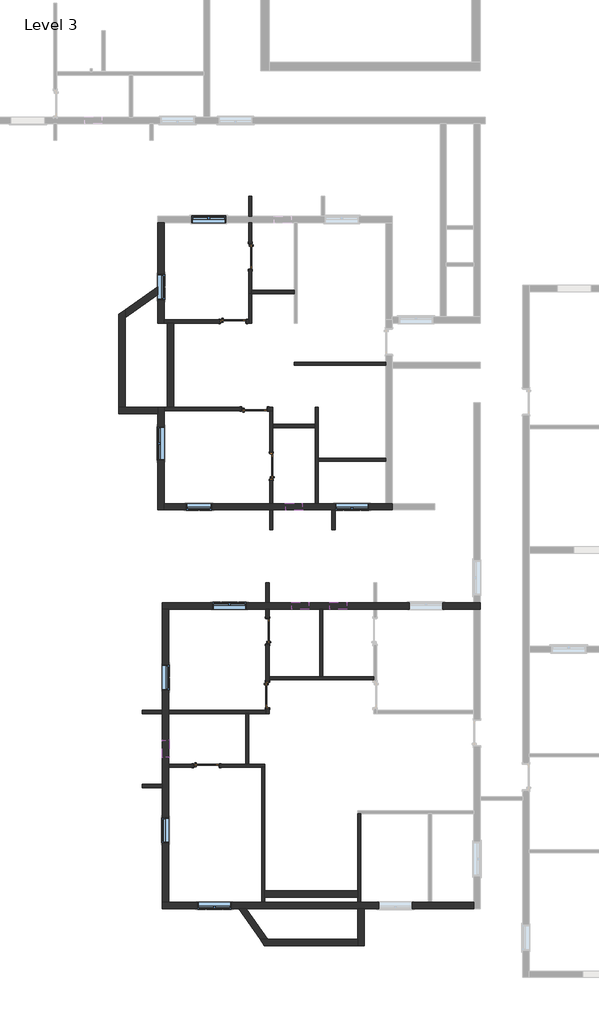
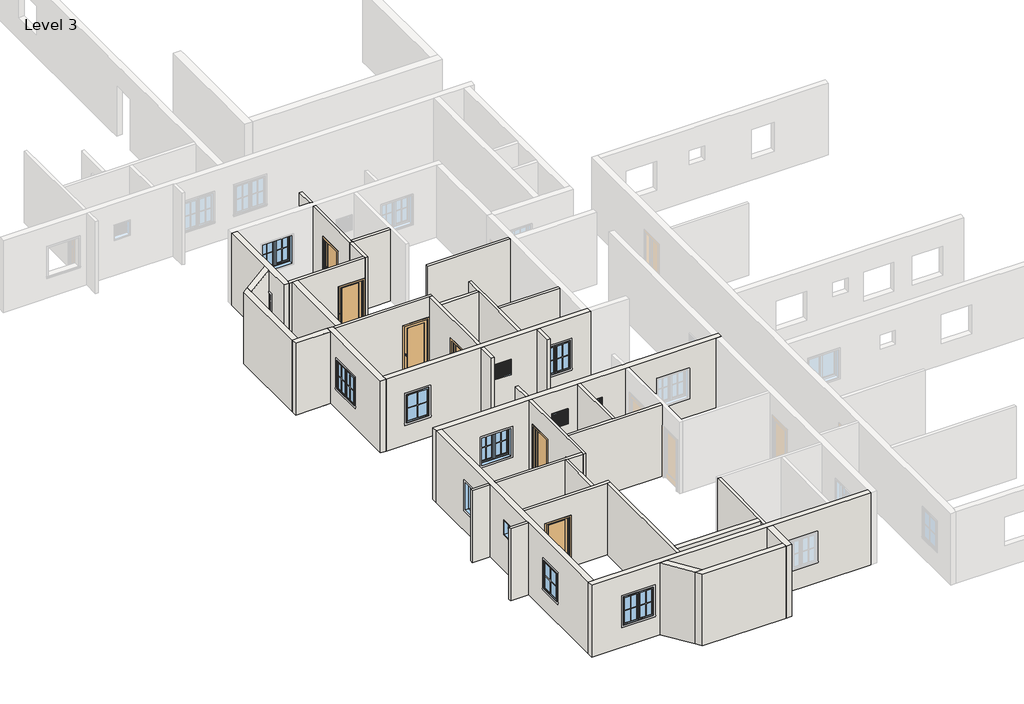
# One storey, part 1 of 7: 39 walls, 13 windows, 7 doors.
"""IFC4 building model written with IfcOpenShell, lengths in millimetres."""

from ifc_helpers import new_model, si_unit, frame, origin, place, context, project, spatial, polyline, outline, extrude, faceted_brep, transform, mapped, element, save
from components import door_3c6ab76a, door_a3feeac7, window_272f20d6, window_casement_double_4_x_4_af3140d2, window_f2d8fef0

model = new_model("IFC4")

# Units and contexts
model_context = context("Model", 3, world=origin())
ifc_project = project(units=[si_unit("LENGTHUNIT", "METRE", prefix="MILLI")], contexts=[model_context])

# Site, building, storey
site = spatial("IfcSite", under=ifc_project)
building = spatial("IfcBuilding", under=site)
storey = spatial("IfcBuildingStorey", under=building, Name="Level 3", Elevation=3200.4)

# Doors
placement = place(None, origin())
door_shape = door_3c6ab76a(model_context)
element("IfcDoor", 1, ObjectType="Door-Interior-Single-1_Panel-Wood : 2'6\" x 7' door", at=placement, inside=storey, context=model_context, shape_type="MappedRepresentation", body=[
    mapped(door_shape, transform((-4216.6759469, -3460.4538828, 3200.4), x_axis=(0.0, -1.0, 0.0), y_axis=(1.0, 0.0, 0.0), z_axis=(0.0, 0.0, 1.0))),
])
element("IfcDoor", 2, ObjectType="Door-Interior-Single-1_Panel-Wood : 2'6\" x 7' door", at=placement, inside=storey, context=model_context, shape_type="MappedRepresentation", body=[
    mapped(door_shape, transform((-5797.8259469, -21840.5288828, 3200.4), x_axis=(1.0, 0.0, 0.0), y_axis=(0.0, 1.0, 0.0), z_axis=(0.0, 0.0, 1.0))),
])
door_2_shape = door_a3feeac7(model_context)
element("IfcDoor", 3, ObjectType="Door-Interior-Single-1_Panel-Wood : 2'6\" x 7' door", at=placement, inside=storey, context=model_context, shape_type="MappedRepresentation", body=[
    mapped(door_2_shape, transform((-3454.6759469, -11032.8288828, 3200.4), x_axis=(0.0, 1.0, 0.0), y_axis=(-1.0, 0.0, 0.0), z_axis=(0.0, 0.0, 1.0))),
])
element("IfcDoor", 4, ObjectType="Door-Interior-Single-1_Panel-Wood : 2'6\" x 7' door", at=placement, inside=storey, context=model_context, shape_type="MappedRepresentation", body=[
    mapped(door_2_shape, transform((-3594.3759469, -16985.9538828, 3200.4), x_axis=(0.0, 1.0, 0.0), y_axis=(-1.0, 0.0, 0.0), z_axis=(0.0, 0.0, 1.0))),
])
element("IfcDoor", 5, ObjectType="Door-Interior-Single-1_Panel-Wood : 36\" x 84\"", at=placement, inside=storey, context=model_context, shape_type="MappedRepresentation", body=[
    mapped(door_shape, transform((-4829.4509469, -5800.4288828, 3200.4), x_axis=(1.0, 0.0, 0.0), y_axis=(0.0, 1.0, 0.0), z_axis=(0.0, 0.0, 1.0))),
])
element("IfcDoor", 6, ObjectType="Door-Interior-Single-1_Panel-Wood : 36\" x 84\"", at=placement, inside=storey, context=model_context, shape_type="MappedRepresentation", body=[
    mapped(door_2_shape, transform((-4067.4509469, -8969.0788828, 3200.4), x_axis=(1.0, 0.0, 0.0), y_axis=(0.0, 1.0, 0.0), z_axis=(0.0, 0.0, 1.0))),
])
element("IfcDoor", 7, ObjectType="Door-Interior-Single-1_Panel-Wood : 36\" x 84\"", at=placement, inside=storey, context=model_context, shape_type="MappedRepresentation", body=[
    mapped(door_2_shape, transform((-3600.7259469, -19291.0038828, 3200.4), x_axis=(0.0, -1.0, 0.0), y_axis=(1.0, 0.0, 0.0), z_axis=(0.0, 0.0, 1.0))),
])

# Walls
element("IfcWall", 8, ObjectType="4.5\" wall", at=placement, inside=storey, context=model_context, shape_type="Brep", body=[
    faceted_brep([(-4277.0009469, -4793.9538828, 6248.4), (-4277.0009469, -2241.2538828, 6248.4), (-4277.0009469, -2241.2538828, 3200.4), (-4277.0009469, -2977.8538828, 3200.4), (-4277.0009469, -2977.8538828, 5359.4), (-4277.0009469, -3943.0538828, 5359.4), (-4277.0009469, -3943.0538828, 3200.4), (-4277.0009469, -4793.9538828, 3200.4), (-4162.7009469, -2241.2538828, 6248.4), (-4162.7009469, -4679.6538828, 6248.4), (-4162.7009469, -4793.9538828, 6248.4), (-4162.7009469, -4793.9538828, 3200.4), (-4162.7009469, -4679.6538828, 3200.4), (-4162.7009469, -3943.0538828, 3200.4), (-4162.7009469, -3943.0538828, 5359.4), (-4162.7009469, -2977.8538828, 5359.4), (-4162.7009469, -2977.8538828, 3200.4), (-4162.7009469, -2241.2538828, 3200.4)], [[[0, 1, 2, 3, 4, 5, 6, 7]], [[8, 9, 10, 11, 12, 13, 14, 15, 16, 17]], [[2, 17, 16, 3]], [[11, 7, 6, 13, 12]], [[1, 0, 10, 9, 8]], [[2, 1, 8, 17]], [[0, 7, 11, 10]], [[5, 14, 13, 6]], [[14, 5, 4, 15]], [[15, 4, 3, 16]]]),
])
element("IfcWall", 9, ObjectType="4.5\" wall", at=placement, inside=storey, context=model_context, shape_type="Brep", body=[
    faceted_brep([(-4277.0009469, -4793.9538828, 3200.4), (-4277.0009469, -5746.4538828, 3200.4), (-4277.0009469, -5860.7538828, 3200.4), (-4277.0009469, -5860.7538828, 6248.4), (-4277.0009469, -5746.4538828, 6248.4), (-4277.0009469, -4793.9538828, 6248.4), (-4162.7009469, -4793.9538828, 3200.4), (-4162.7009469, -4793.9538828, 6248.4), (-4162.7009469, -5860.7538828, 6248.4), (-4162.7009469, -5860.7538828, 3200.4)], [[[0, 1, 2, 3, 4, 5]], [[6, 7, 8, 9]], [[2, 1, 0, 6, 9]], [[5, 4, 3, 8, 7]], [[0, 5, 7, 6]], [[3, 2, 9, 8]]]),
])
element("IfcWall", 10, ObjectType="4.5\" wall", at=placement, inside=storey, context=model_context, shape_type="Brep", body=[
    faceted_brep([(-7325.0009469, -5746.4538828, 6248.4), (-4277.0009469, -5746.4538828, 6248.4), (-4277.0009469, -5746.4538828, 3200.4), (-4346.8509469, -5746.4538828, 3200.4), (-4346.8509469, -5746.4538828, 5359.4), (-5312.0509469, -5746.4538828, 5359.4), (-5312.0509469, -5746.4538828, 3200.4), (-7325.0009469, -5746.4538828, 3200.4), (-4277.0009469, -5860.7538828, 6248.4), (-6982.1009469, -5860.7538828, 6248.4), (-7210.7009469, -5860.7538828, 6248.4), (-7325.0009469, -5860.7538828, 6248.4), (-7325.0009469, -5860.7538828, 3200.4), (-7210.7009469, -5860.7538828, 3200.4), (-6982.1009469, -5860.7538828, 3200.4), (-5312.0509469, -5860.7538828, 3200.4), (-5312.0509469, -5860.7538828, 5359.4), (-4346.8509469, -5860.7538828, 5359.4), (-4346.8509469, -5860.7538828, 3200.4), (-4277.0009469, -5860.7538828, 3200.4)], [[[0, 1, 2, 3, 4, 5, 6, 7]], [[8, 9, 10, 11, 12, 13, 14, 15, 16, 17, 18, 19]], [[12, 7, 6, 15, 14, 13]], [[2, 19, 18, 3]], [[1, 0, 11, 10, 9, 8]], [[0, 7, 12, 11]], [[2, 1, 8, 19]], [[17, 4, 3, 18]], [[4, 17, 16, 5]], [[5, 16, 15, 6]]]),
])
element("IfcWall", 11, ObjectType="4.5\" wall", at=placement, inside=storey, context=model_context, shape_type="SweptSolid", body=[
    extrude(outline(polyline([(-2638.7009469, -4793.9538828), (-4162.7009469, -4793.9538828), (-4162.7009469, -4679.6538828), (-2638.7009469, -4679.6538828), (-2638.7009469, -4793.9538828)])), frame((0.0, 0.0, 3200.4), z_axis=(0.0, 0.0, 1.0), x_axis=(1.0, 0.0, 0.0)), (0.0, 0.0, 1.0), 3048.0),
])
element("IfcWall", 12, ObjectType="4.5\" wall", at=placement, inside=storey, context=model_context, shape_type="SweptSolid", body=[
    extrude(outline(polyline([(-2638.7009469, -7270.4538828), (675.9990531, -7270.4538828), (675.9990531, -7384.7538828), (-2638.7009469, -7384.7538828), (-2638.7009469, -7270.4538828)])), frame((0.0, 0.0, 3200.4), z_axis=(0.0, 0.0, 1.0), x_axis=(1.0, 0.0, 0.0)), (0.0, 0.0, 1.0), 3048.0),
])
element("IfcWall", 13, ObjectType="4.5\" wall", at=placement, inside=storey, context=model_context, shape_type="Brep", body=[
    faceted_brep([(-7325.0009469, -8908.7538828, 6248.4), (-7210.7009469, -8908.7538828, 6248.4), (-6982.1009469, -8908.7538828, 6248.4), (-3400.7009469, -8908.7538828, 6248.4), (-3400.7009469, -8908.7538828, 3200.4), (-3584.8509469, -8908.7538828, 3200.4), (-3584.8509469, -8908.7538828, 5359.4), (-4550.0509469, -8908.7538828, 5359.4), (-4550.0509469, -8908.7538828, 3200.4), (-6982.1009469, -8908.7538828, 3200.4), (-7210.7009469, -8908.7538828, 3200.4), (-7325.0009469, -8908.7538828, 3200.4), (-3400.7009469, -9023.0538828, 6248.4), (-3515.0009469, -9023.0538828, 6248.4), (-7325.0009469, -9023.0538828, 6248.4), (-7325.0009469, -9023.0538828, 3200.4), (-4550.0509469, -9023.0538828, 3200.4), (-4550.0509469, -9023.0538828, 5359.4), (-3584.8509469, -9023.0538828, 5359.4), (-3584.8509469, -9023.0538828, 3200.4), (-3515.0009469, -9023.0538828, 3200.4), (-3400.7009469, -9023.0538828, 3200.4)], [[[0, 1, 2, 3, 4, 5, 6, 7, 8, 9, 10, 11]], [[12, 13, 14, 15, 16, 17, 18, 19, 20, 21]], [[4, 21, 20, 19, 5]], [[15, 11, 10, 9, 8, 16]], [[3, 2, 1, 0, 14, 13, 12]], [[4, 3, 12, 21]], [[0, 11, 15, 14]], [[18, 6, 5, 19]], [[6, 18, 17, 7]], [[7, 17, 16, 8]]]),
])
element("IfcWall", 14, ObjectType="4.5\" wall", at=placement, inside=storey, context=model_context, shape_type="SweptSolid", body=[
    extrude(outline(polyline([(-1876.7009469, -9632.6538828), (-3400.7009469, -9632.6538828), (-3400.7009469, -9518.3538828), (-1876.7009469, -9518.3538828), (-1876.7009469, -9632.6538828)])), frame((0.0, 0.0, 3200.4), z_axis=(0.0, 0.0, 1.0), x_axis=(1.0, 0.0, 0.0)), (0.0, 0.0, 1.0), 3048.0),
])
element("IfcWall", 15, ObjectType="4.5\" wall", at=placement, inside=storey, context=model_context, shape_type="Brep", body=[
    faceted_brep([(-1762.4009469, -12375.8538828, 3200.4), (-1762.4009469, -10851.8538828, 3200.4), (-1762.4009469, -10737.5538828, 3200.4), (-1762.4009469, -8908.7538828, 3200.4), (-1762.4009469, -8908.7538828, 6248.4), (-1762.4009469, -10737.5538828, 6248.4), (-1762.4009469, -10851.8538828, 6248.4), (-1762.4009469, -12375.8538828, 6248.4), (-1876.7009469, -12375.8538828, 3200.4), (-1876.7009469, -12375.8538828, 6248.4), (-1876.7009469, -9632.6538828, 6248.4), (-1876.7009469, -9518.3538828, 6248.4), (-1876.7009469, -8908.7538828, 6248.4), (-1876.7009469, -8908.7538828, 3200.4), (-1876.7009469, -9518.3538828, 3200.4), (-1876.7009469, -9632.6538828, 3200.4)], [[[0, 1, 2, 3, 4, 5, 6, 7]], [[8, 9, 10, 11, 12, 13, 14, 15]], [[3, 2, 1, 0, 8, 15, 14, 13]], [[4, 3, 13, 12]], [[7, 6, 5, 4, 12, 11, 10, 9]], [[0, 7, 9, 8]]]),
])
element("IfcWall", 16, ObjectType="4.5\" wall", at=placement, inside=storey, context=model_context, shape_type="Brep", body=[
    faceted_brep([(-3400.7009469, -9023.0538828, 6248.4), (-3400.7009469, -9518.3538828, 6248.4), (-3400.7009469, -9632.6538828, 6248.4), (-3400.7009469, -12375.8538828, 6248.4), (-3400.7009469, -12375.8538828, 3200.4), (-3400.7009469, -11515.4288828, 3200.4), (-3400.7009469, -11515.4288828, 5359.4), (-3400.7009469, -10550.2288828, 5359.4), (-3400.7009469, -10550.2288828, 3200.4), (-3400.7009469, -9632.6538828, 3200.4), (-3400.7009469, -9518.3538828, 3200.4), (-3400.7009469, -9023.0538828, 3200.4), (-3515.0009469, -12375.8538828, 6248.4), (-3515.0009469, -9023.0538828, 6248.4), (-3515.0009469, -9023.0538828, 3200.4), (-3515.0009469, -10550.2288828, 3200.4), (-3515.0009469, -10550.2288828, 5359.4), (-3515.0009469, -11515.4288828, 5359.4), (-3515.0009469, -11515.4288828, 3200.4), (-3515.0009469, -12375.8538828, 3200.4)], [[[0, 1, 2, 3, 4, 5, 6, 7, 8, 9, 10, 11]], [[12, 13, 14, 15, 16, 17, 18, 19]], [[4, 19, 18, 5]], [[14, 11, 10, 9, 8, 15]], [[3, 2, 1, 0, 13, 12]], [[4, 3, 12, 19]], [[0, 11, 14, 13]], [[7, 16, 15, 8]], [[16, 7, 6, 17]], [[17, 6, 5, 18]]]),
])
element("IfcWall", 17, ObjectType="4.5\" wall", at=placement, inside=storey, context=model_context, shape_type="SweptSolid", body=[
    extrude(outline(polyline([(-1762.4009469, -10737.5538828), (675.9990531, -10737.5538828), (675.9990531, -10851.8538828), (-1762.4009469, -10851.8538828), (-1762.4009469, -10737.5538828)])), frame((0.0, 0.0, 3200.4), z_axis=(0.0, 0.0, 1.0), x_axis=(1.0, 0.0, 0.0)), (0.0, 0.0, 1.0), 3048.0),
])
element("IfcWall", 18, ObjectType="4.5\" wall", at=placement, inside=storey, context=model_context, shape_type="SweptSolid", body=[
    extrude(outline(polyline([(-3515.0009469, -13328.3538828), (-3515.0009469, -12604.4538828), (-3400.7009469, -12604.4538828), (-3400.7009469, -13328.3538828), (-3515.0009469, -13328.3538828)])), frame((0.0, 0.0, 3200.4), z_axis=(0.0, 0.0, 1.0), x_axis=(1.0, 0.0, 0.0)), (0.0, 0.0, 1.0), 3048.0),
])
element("IfcWall", 19, ObjectType="4.5\" wall", at=placement, inside=storey, context=model_context, shape_type="SweptSolid", body=[
    extrude(outline(polyline([(-1152.8009469, -12604.4538828), (-1152.8009469, -13328.3538828), (-1267.1009469, -13328.3538828), (-1267.1009469, -12604.4538828), (-1152.8009469, -12604.4538828)])), frame((0.0, 0.0, 3200.4), z_axis=(0.0, 0.0, 1.0), x_axis=(1.0, 0.0, 0.0)), (0.0, 0.0, 1.0), 3048.0),
])
element("IfcWall", 20, ObjectType="4.5\" wall", at=placement, inside=storey, context=model_context, shape_type="SweptSolid", body=[
    extrude(outline(polyline([(-4162.7009469, -1288.7538828), (-4162.7009469, -2012.6538828), (-4277.0009469, -2012.6538828), (-4277.0009469, -1288.7538828), (-4162.7009469, -1288.7538828)])), frame((0.0, 0.0, 3200.4), z_axis=(0.0, 0.0, 1.0), x_axis=(1.0, 0.0, 0.0)), (0.0, 0.0, 1.0), 3048.0),
])
element("IfcWall", 21, ObjectType="4.5\" wall", at=placement, inside=storey, context=model_context, shape_type="Brep", body=[
    faceted_brep([(231.4990531, -18624.2538828, 3200.4), (-1597.3009469, -18624.2538828, 3200.4), (-1711.6009469, -18624.2538828, 3200.4), (-3540.4009469, -18624.2538828, 3200.4), (-3540.4009469, -18624.2538828, 6248.4), (-1711.6009469, -18624.2538828, 6248.4), (-1597.3009469, -18624.2538828, 6248.4), (231.4990531, -18624.2538828, 6248.4), (231.4990531, -18738.5538828, 3200.4), (231.4990531, -18738.5538828, 6248.4), (-3540.4009469, -18738.5538828, 6248.4), (-3540.4009469, -18738.5538828, 3200.4)], [[[0, 1, 2, 3, 4, 5, 6, 7]], [[8, 9, 10, 11]], [[3, 2, 1, 0, 8, 11]], [[7, 6, 5, 4, 10, 9]], [[4, 3, 11, 10]], [[0, 7, 9, 8]]]),
])
element("IfcWall", 22, ObjectType="4.5\" wall", at=placement, inside=storey, context=model_context, shape_type="SweptSolid", body=[
    extrude(outline(polyline([(-1597.3009469, -16185.8538828), (-1597.3009469, -18624.2538828), (-1711.6009469, -18624.2538828), (-1711.6009469, -16185.8538828), (-1597.3009469, -16185.8538828)])), frame((0.0, 0.0, 3200.4), z_axis=(0.0, 0.0, 1.0), x_axis=(1.0, 0.0, 0.0)), (0.0, 0.0, 1.0), 3048.0),
])
element("IfcWall", 23, ObjectType="4.5\" wall", at=placement, inside=storey, context=model_context, shape_type="SweptSolid", body=[
    extrude(outline(polyline([(-3540.4009469, -15233.3538828), (-3540.4009469, -15957.2538828), (-3654.7009469, -15957.2538828), (-3654.7009469, -15233.3538828), (-3540.4009469, -15233.3538828)])), frame((0.0, 0.0, 3200.4), z_axis=(0.0, 0.0, 1.0), x_axis=(1.0, 0.0, 0.0)), (0.0, 0.0, 1.0), 3048.0),
])
element("IfcWall", 24, ObjectType="4.5\" wall", at=placement, inside=storey, context=model_context, shape_type="Brep", body=[
    faceted_brep([(-3654.7009469, -19957.7538828, 6248.4), (-3654.7009469, -19843.4538828, 6248.4), (-3654.7009469, -16185.8538828, 6248.4), (-3654.7009469, -16185.8538828, 3200.4), (-3654.7009469, -16503.3538828, 3200.4), (-3654.7009469, -16503.3538828, 5359.4), (-3654.7009469, -17468.5538828, 5359.4), (-3654.7009469, -17468.5538828, 3200.4), (-3654.7009469, -18808.4038828, 3200.4), (-3654.7009469, -18808.4038828, 5359.4), (-3654.7009469, -19773.6038828, 5359.4), (-3654.7009469, -19773.6038828, 3200.4), (-3654.7009469, -19843.4538828, 3200.4), (-3654.7009469, -19957.7538828, 3200.4), (-3540.4009469, -16185.8538828, 6248.4), (-3540.4009469, -18624.2538828, 6248.4), (-3540.4009469, -18738.5538828, 6248.4), (-3540.4009469, -19957.7538828, 6248.4), (-3540.4009469, -19957.7538828, 3200.4), (-3540.4009469, -19773.6038828, 3200.4), (-3540.4009469, -19773.6038828, 5359.4), (-3540.4009469, -18808.4038828, 5359.4), (-3540.4009469, -18808.4038828, 3200.4), (-3540.4009469, -18738.5538828, 3200.4), (-3540.4009469, -18624.2538828, 3200.4), (-3540.4009469, -17468.5538828, 3200.4), (-3540.4009469, -17468.5538828, 5359.4), (-3540.4009469, -16503.3538828, 5359.4), (-3540.4009469, -16503.3538828, 3200.4), (-3540.4009469, -16185.8538828, 3200.4)], [[[0, 1, 2, 3, 4, 5, 6, 7, 8, 9, 10, 11, 12, 13]], [[14, 15, 16, 17, 18, 19, 20, 21, 22, 23, 24, 25, 26, 27, 28, 29]], [[3, 29, 28, 4]], [[18, 13, 12, 11, 19]], [[7, 25, 24, 23, 22, 8]], [[2, 1, 0, 17, 16, 15, 14]], [[3, 2, 14, 29]], [[0, 13, 18, 17]], [[27, 5, 4, 28]], [[5, 27, 26, 6]], [[6, 26, 25, 7]], [[10, 20, 19, 11]], [[20, 10, 9, 21]], [[21, 9, 8, 22]]]),
])
element("IfcWall", 25, ObjectType="4.5\" wall", at=placement, inside=storey, context=model_context, shape_type="Brep", body=[
    faceted_brep([(-3654.7009469, -19843.4538828, 3200.4), (-7159.9009469, -19843.4538828, 3200.4), (-7159.9009469, -19843.4538828, 6248.4), (-3654.7009469, -19843.4538828, 6248.4), (-3654.7009469, -19957.7538828, 3200.4), (-3654.7009469, -19957.7538828, 6248.4), (-4264.3009469, -19957.7538828, 6248.4), (-4378.6009469, -19957.7538828, 6248.4), (-7159.9009469, -19957.7538828, 6248.4), (-7159.9009469, -19957.7538828, 3200.4), (-4378.6009469, -19957.7538828, 3200.4), (-4264.3009469, -19957.7538828, 3200.4)], [[[0, 1, 2, 3]], [[4, 5, 6, 7, 8, 9, 10, 11]], [[1, 0, 4, 11, 10, 9]], [[3, 2, 8, 7, 6, 5]], [[2, 1, 9, 8]], [[0, 3, 5, 4]]]),
])
element("IfcWall", 26, ObjectType="4.5\" wall", at=placement, inside=storey, context=model_context, shape_type="Brep", body=[
    faceted_brep([(-7159.9009469, -21786.5538828, 6248.4), (-4378.6009469, -21786.5538828, 6248.4), (-4264.3009469, -21786.5538828, 6248.4), (-3692.8009469, -21786.5538828, 6248.4), (-3692.8009469, -21786.5538828, 3200.4), (-4264.3009469, -21786.5538828, 3200.4), (-4378.6009469, -21786.5538828, 3200.4), (-5315.2259469, -21786.5538828, 3200.4), (-5315.2259469, -21786.5538828, 5359.4), (-6280.4259469, -21786.5538828, 5359.4), (-6280.4259469, -21786.5538828, 3200.4), (-7159.9009469, -21786.5538828, 3200.4), (-3692.8009469, -21900.8538828, 6248.4), (-3807.1009469, -21900.8538828, 6248.4), (-7159.9009469, -21900.8538828, 6248.4), (-7159.9009469, -21900.8538828, 3200.4), (-6280.4259469, -21900.8538828, 3200.4), (-6280.4259469, -21900.8538828, 5359.4), (-5315.2259469, -21900.8538828, 5359.4), (-5315.2259469, -21900.8538828, 3200.4), (-3807.1009469, -21900.8538828, 3200.4), (-3692.8009469, -21900.8538828, 3200.4)], [[[0, 1, 2, 3, 4, 5, 6, 7, 8, 9, 10, 11]], [[12, 13, 14, 15, 16, 17, 18, 19, 20, 21]], [[15, 11, 10, 16]], [[4, 21, 20, 19, 7, 6, 5]], [[3, 2, 1, 0, 14, 13, 12]], [[0, 11, 15, 14]], [[4, 3, 12, 21]], [[18, 8, 7, 19]], [[8, 18, 17, 9]], [[9, 17, 16, 10]]]),
])
element("IfcWall", 27, ObjectType="4.5\" wall", at=placement, inside=storey, context=model_context, shape_type="Brep", body=[
    faceted_brep([(-3692.8009469, -26777.6538828, 3200.4), (-3692.8009469, -26587.1538828, 3200.4), (-3692.8009469, -26358.5538828, 3200.4), (-3692.8009469, -21900.8538828, 3200.4), (-3692.8009469, -21900.8538828, 6248.4), (-3692.8009469, -26358.5538828, 6248.4), (-3692.8009469, -26587.1538828, 6248.4), (-3692.8009469, -26777.6538828, 6248.4), (-3807.1009469, -26777.6538828, 3200.4), (-3807.1009469, -26777.6538828, 6248.4), (-3807.1009469, -21900.8538828, 6248.4), (-3807.1009469, -21900.8538828, 3200.4)], [[[0, 1, 2, 3, 4, 5, 6, 7]], [[8, 9, 10, 11]], [[3, 2, 1, 0, 8, 11]], [[7, 6, 5, 4, 10, 9]], [[4, 3, 11, 10]], [[0, 7, 9, 8]]]),
])
element("IfcWall", 28, ObjectType="4.5\" wall", at=placement, inside=storey, context=model_context, shape_type="SweptSolid", body=[
    extrude(outline(polyline([(-7388.5009469, -22629.8863256), (-8112.4009469, -22629.8863256), (-8112.4009469, -22515.5863256), (-7388.5009469, -22515.5863256), (-7388.5009469, -22629.8863256)])), frame((0.0, 0.0, 3200.4), z_axis=(0.0, 0.0, 1.0), x_axis=(1.0, 0.0, 0.0)), (0.0, 0.0, 1.0), 3048.0),
])
element("IfcWall", 29, ObjectType="4.5\" wall", at=placement, inside=storey, context=model_context, shape_type="SweptSolid", body=[
    extrude(outline(polyline([(-8112.4009469, -19843.4538828), (-7388.5009469, -19843.4538828), (-7388.5009469, -19957.7538828), (-8112.4009469, -19957.7538828), (-8112.4009469, -19843.4538828)])), frame((0.0, 0.0, 3200.4), z_axis=(0.0, 0.0, 1.0), x_axis=(1.0, 0.0, 0.0)), (0.0, 0.0, 1.0), 3048.0),
])
element("IfcWall", 30, ObjectType="4.5\" wall", at=placement, inside=storey, context=model_context, shape_type="SweptSolid", body=[
    extrude(outline(polyline([(-4378.6009469, -21786.5538828), (-4378.6009469, -19957.7538828), (-4264.3009469, -19957.7538828), (-4264.3009469, -21786.5538828), (-4378.6009469, -21786.5538828)])), frame((0.0, 0.0, 3200.4), z_axis=(0.0, 0.0, 1.0), x_axis=(1.0, 0.0, 0.0)), (0.0, 0.0, 1.0), 3048.0),
])
element("IfcWall", 31, ObjectType="4.5\" wall", at=placement, inside=storey, context=model_context, shape_type="Brep", body=[
    faceted_brep([(-340.0009469, -23577.2538828, 3200.4), (-340.0009469, -26358.5538828, 3200.4), (-340.0009469, -26587.1538828, 3200.4), (-340.0009469, -26777.6538828, 3200.4), (-340.0009469, -26777.6538828, 6248.4), (-340.0009469, -26587.1538828, 6248.4), (-340.0009469, -26358.5538828, 6248.4), (-340.0009469, -23577.2538828, 6248.4), (-225.7009469, -23577.2538828, 3200.4), (-225.7009469, -23577.2538828, 6248.4), (-225.7009469, -26777.6538828, 6248.4), (-225.7009469, -26777.6538828, 3200.4)], [[[0, 1, 2, 3, 4, 5, 6, 7]], [[8, 9, 10, 11]], [[3, 2, 1, 0, 8, 11]], [[7, 6, 5, 4, 10, 9]], [[0, 7, 9, 8]], [[4, 3, 11, 10]]]),
])
element("IfcWall", 32, ObjectType="9\"", at=placement, inside=storey, context=model_context, shape_type="Brep", body=[
    faceted_brep([(-7553.6009469, -2241.2538828, 3200.4), (-7553.6009469, -4556.8220214, 3200.4), (-7553.6009469, -4835.8638828, 3200.4), (-7553.6009469, -5860.7538828, 3200.4), (-7553.6009469, -5860.7538828, 6248.4), (-7553.6009469, -4835.8638828, 6248.4), (-7553.6009469, -4556.8220214, 6248.4), (-7553.6009469, -2241.2538828, 6248.4), (-7553.6009469, -5016.2038828, 5334.0), (-7553.6009469, -5016.2038828, 4114.8), (-7553.6009469, -4101.8038828, 4114.8), (-7553.6009469, -4101.8038828, 5334.0), (-7325.0009469, -2241.2538828, 3200.4), (-7325.0009469, -2241.2538828, 6248.4), (-7325.0009469, -5746.4538828, 6248.4), (-7325.0009469, -5860.7538828, 6248.4), (-7325.0009469, -5860.7538828, 3200.4), (-7325.0009469, -5746.4538828, 3200.4), (-7325.0009469, -5016.2038828, 5334.0), (-7325.0009469, -4101.8038828, 5334.0), (-7325.0009469, -4101.8038828, 4114.8), (-7325.0009469, -5016.2038828, 4114.8)], [[[0, 1, 2, 3, 4, 5, 6, 7], [8, 9, 10, 11]], [[12, 13, 14, 15, 16, 17], [18, 19, 20, 21]], [[3, 2, 1, 0, 12, 17, 16]], [[7, 6, 5, 4, 15, 14, 13]], [[0, 7, 13, 12]], [[4, 3, 16, 15]], [[9, 8, 18, 21]], [[10, 9, 21, 20]], [[11, 10, 20, 19]], [[8, 11, 19, 18]]]),
])
element("IfcWall", 33, ObjectType="9\"", at=placement, inside=storey, context=model_context, shape_type="SweptSolid", body=[
    extrude(outline(polyline([(-6982.1009469, -5860.7538828), (-6982.1009469, -8908.7538828), (-7210.7009469, -8908.7538828), (-7210.7009469, -5860.7538828), (-6982.1009469, -5860.7538828)])), frame((0.0, 0.0, 3200.4), z_axis=(0.0, 0.0, 1.0), x_axis=(1.0, 0.0, 0.0)), (0.0, 0.0, 1.0), 3048.0),
])
element("IfcWall", 34, ObjectType="9\"", at=placement, inside=storey, context=model_context, shape_type="Brep", body=[
    faceted_brep([(-7553.6009469, -8908.7538828, 3200.4), (-7553.6009469, -9137.3538828, 3200.4), (-7553.6009469, -12604.4538828, 3200.4), (-7553.6009469, -12604.4538828, 6248.4), (-7553.6009469, -9137.3538828, 6248.4), (-7553.6009469, -8908.7538828, 6248.4), (-7553.6009469, -9600.9038828, 5334.0), (-7553.6009469, -10820.1038828, 5334.0), (-7553.6009469, -10820.1038828, 4114.8), (-7553.6009469, -9600.9038828, 4114.8), (-7325.0009469, -8908.7538828, 3200.4), (-7325.0009469, -8908.7538828, 6248.4), (-7325.0009469, -9023.0538828, 6248.4), (-7325.0009469, -12375.8538828, 6248.4), (-7325.0009469, -12604.4538828, 6248.4), (-7325.0009469, -12604.4538828, 3200.4), (-7325.0009469, -12375.8538828, 3200.4), (-7325.0009469, -9023.0538828, 3200.4), (-7325.0009469, -9600.9038828, 5334.0), (-7325.0009469, -9600.9038828, 4114.8), (-7325.0009469, -10820.1038828, 4114.8), (-7325.0009469, -10820.1038828, 5334.0)], [[[0, 1, 2, 3, 4, 5], [6, 7, 8, 9]], [[10, 11, 12, 13, 14, 15, 16, 17], [18, 19, 20, 21]], [[2, 1, 0, 10, 17, 16, 15]], [[5, 4, 3, 14, 13, 12, 11]], [[3, 2, 15, 14]], [[0, 5, 11, 10]], [[19, 18, 6, 9]], [[20, 19, 9, 8]], [[21, 20, 8, 7]], [[18, 21, 7, 6]]]),
])
element("IfcWall", 35, ObjectType="9\"", at=placement, inside=storey, context=model_context, shape_type="Brep", body=[
    faceted_brep([(-7325.0009469, -12604.4538828, 3200.4), (-3515.0009469, -12604.4538828, 3200.4), (-3400.7009469, -12604.4538828, 3200.4), (-1267.1009469, -12604.4538828, 3200.4), (-1152.8009469, -12604.4538828, 3200.4), (904.5990531, -12604.4538828, 3200.4), (904.5990531, -12604.4538828, 6248.4), (-1152.8009469, -12604.4538828, 6248.4), (-1267.1009469, -12604.4538828, 6248.4), (-3400.7009469, -12604.4538828, 6248.4), (-3515.0009469, -12604.4538828, 6248.4), (-7325.0009469, -12604.4538828, 6248.4), (-2333.9009469, -12604.4538828, 5334.0), (-2333.9009469, -12604.4538828, 4724.4), (-2943.5009469, -12604.4538828, 4724.4), (-2943.5009469, -12604.4538828, 5334.0), (-6524.9009469, -12604.4538828, 5334.0), (-5610.5009469, -12604.4538828, 5334.0), (-5610.5009469, -12604.4538828, 4114.8), (-6524.9009469, -12604.4538828, 4114.8), (-1152.8009469, -12604.4538828, 5334.0), (66.3990531, -12604.4538828, 5334.0), (66.3990531, -12604.4538828, 4114.8), (-1152.8009469, -12604.4538828, 4114.8), (-7325.0009469, -12375.8538828, 3200.4), (-7325.0009469, -12375.8538828, 6248.4), (-3515.0009469, -12375.8538828, 6248.4), (-3400.7009469, -12375.8538828, 6248.4), (-1876.7009469, -12375.8538828, 6248.4), (-1762.4009469, -12375.8538828, 6248.4), (675.9990531, -12375.8538828, 6248.4), (904.5990531, -12375.8538828, 6248.4), (904.5990531, -12375.8538828, 3200.4), (675.9990531, -12375.8538828, 3200.4), (-1762.4009469, -12375.8538828, 3200.4), (-1876.7009469, -12375.8538828, 3200.4), (-3400.7009469, -12375.8538828, 3200.4), (-3515.0009469, -12375.8538828, 3200.4), (-2333.9009469, -12375.8538828, 5334.0), (-2943.5009469, -12375.8538828, 5334.0), (-2943.5009469, -12375.8538828, 4724.4), (-2333.9009469, -12375.8538828, 4724.4), (-6524.9009469, -12375.8538828, 5334.0), (-6524.9009469, -12375.8538828, 4114.8), (-5610.5009469, -12375.8538828, 4114.8), (-5610.5009469, -12375.8538828, 5334.0), (-1152.8009469, -12375.8538828, 5334.0), (-1152.8009469, -12375.8538828, 4114.8), (66.3990531, -12375.8538828, 4114.8), (66.3990531, -12375.8538828, 5334.0)], [[[0, 1, 2, 3, 4, 5, 6, 7, 8, 9, 10, 11], [12, 13, 14, 15], [16, 17, 18, 19], [20, 21, 22, 23]], [[24, 25, 26, 27, 28, 29, 30, 31, 32, 33, 34, 35, 36, 37], [38, 39, 40, 41], [42, 43, 44, 45], [46, 47, 48, 49]], [[5, 4, 3, 2, 1, 0, 24, 37, 36, 35, 34, 33, 32]], [[11, 10, 9, 8, 7, 6, 31, 30, 29, 28, 27, 26, 25]], [[0, 11, 25, 24]], [[6, 5, 32, 31]], [[13, 12, 38, 41]], [[14, 13, 41, 40]], [[15, 14, 40, 39]], [[12, 15, 39, 38]], [[43, 42, 16, 19]], [[44, 43, 19, 18]], [[45, 44, 18, 17]], [[42, 45, 17, 16]], [[47, 46, 20, 23]], [[48, 47, 23, 22]], [[49, 48, 22, 21]], [[46, 49, 21, 20]]]),
])
element("IfcWall", 36, ObjectType="9\"", at=placement, inside=storey, context=model_context, shape_type="SweptSolid", body=[
    extrude(outline(polyline([(-7820.3009469, -8908.7538828), (-7553.6009469, -8908.7538828), (-7553.6009469, -9137.3538828), (-7820.3009469, -9137.3538828), (-7820.3009469, -8908.7538828)])), frame((0.0, 0.0, 3200.4), z_axis=(0.0, 0.0, 1.0), x_axis=(1.0, 0.0, 0.0)), (0.0, 0.0, 1.0), 3048.0),
])
element("IfcWall", 37, ObjectType="9\"", at=placement, inside=storey, context=model_context, shape_type="Brep", body=[
    faceted_brep([(-7388.5009469, -16185.8538828, 3200.4), (-7159.9009469, -16185.8538828, 3200.4), (-3654.7009469, -16185.8538828, 3200.4), (-3540.4009469, -16185.8538828, 3200.4), (-1711.6009469, -16185.8538828, 3200.4), (-1597.3009469, -16185.8538828, 3200.4), (231.4990531, -16185.8538828, 3200.4), (345.7990531, -16185.8538828, 3200.4), (3850.9990531, -16185.8538828, 3200.4), (4079.5990531, -16185.8538828, 3200.4), (4079.5990531, -16185.8538828, 6248.4), (3850.9990531, -16185.8538828, 6248.4), (345.7990531, -16185.8538828, 6248.4), (231.4990531, -16185.8538828, 6248.4), (-1597.3009469, -16185.8538828, 6248.4), (-1711.6009469, -16185.8538828, 6248.4), (-3540.4009469, -16185.8538828, 6248.4), (-3654.7009469, -16185.8538828, 6248.4), (-7159.9009469, -16185.8538828, 6248.4), (-7388.5009469, -16185.8538828, 6248.4), (-740.0509469, -16185.8538828, 5334.0), (-740.0509469, -16185.8538828, 4724.4), (-1349.6509469, -16185.8538828, 4724.4), (-1349.6509469, -16185.8538828, 5334.0), (-2111.6509469, -16185.8538828, 5334.0), (-2111.6509469, -16185.8538828, 4724.4), (-2721.2509469, -16185.8538828, 4724.4), (-2721.2509469, -16185.8538828, 5334.0), (2736.5740531, -16185.8538828, 5334.0), (2736.5740531, -16185.8538828, 4114.8), (1517.3740531, -16185.8538828, 4114.8), (1517.3740531, -16185.8538828, 5334.0), (-4359.5509469, -16185.8538828, 5334.0), (-4359.5509469, -16185.8538828, 4114.8), (-5578.7509469, -16185.8538828, 4114.8), (-5578.7509469, -16185.8538828, 5334.0), (-7388.5009469, -15957.2538828, 3200.4), (-7388.5009469, -15957.2538828, 6248.4), (-3654.7009469, -15957.2538828, 6248.4), (-3540.4009469, -15957.2538828, 6248.4), (231.4990531, -15957.2538828, 6248.4), (345.7990531, -15957.2538828, 6248.4), (3850.9990531, -15957.2538828, 6248.4), (4079.5990531, -15957.2538828, 6248.4), (4079.5990531, -15957.2538828, 3200.4), (3850.9990531, -15957.2538828, 3200.4), (345.7990531, -15957.2538828, 3200.4), (231.4990531, -15957.2538828, 3200.4), (-3540.4009469, -15957.2538828, 3200.4), (-3654.7009469, -15957.2538828, 3200.4), (-740.0509469, -15957.2538828, 5334.0), (-1349.6509469, -15957.2538828, 5334.0), (-1349.6509469, -15957.2538828, 4724.4), (-740.0509469, -15957.2538828, 4724.4), (-2111.6509469, -15957.2538828, 5334.0), (-2721.2509469, -15957.2538828, 5334.0), (-2721.2509469, -15957.2538828, 4724.4), (-2111.6509469, -15957.2538828, 4724.4), (2736.5740531, -15957.2538828, 5334.0), (1517.3740531, -15957.2538828, 5334.0), (1517.3740531, -15957.2538828, 4114.8), (2736.5740531, -15957.2538828, 4114.8), (-4359.5509469, -15957.2538828, 5334.0), (-5578.7509469, -15957.2538828, 5334.0), (-5578.7509469, -15957.2538828, 4114.8), (-4359.5509469, -15957.2538828, 4114.8)], [[[0, 1, 2, 3, 4, 5, 6, 7, 8, 9, 10, 11, 12, 13, 14, 15, 16, 17, 18, 19], [20, 21, 22, 23], [24, 25, 26, 27], [28, 29, 30, 31], [32, 33, 34, 35]], [[36, 37, 38, 39, 40, 41, 42, 43, 44, 45, 46, 47, 48, 49], [50, 51, 52, 53], [54, 55, 56, 57], [58, 59, 60, 61], [62, 63, 64, 65]], [[9, 8, 7, 6, 5, 4, 3, 2, 1, 0, 36, 49, 48, 47, 46, 45, 44]], [[19, 18, 17, 16, 15, 14, 13, 12, 11, 10, 43, 42, 41, 40, 39, 38, 37]], [[0, 19, 37, 36]], [[10, 9, 44, 43]], [[21, 20, 50, 53]], [[22, 21, 53, 52]], [[23, 22, 52, 51]], [[20, 23, 51, 50]], [[25, 24, 54, 57]], [[26, 25, 57, 56]], [[27, 26, 56, 55]], [[24, 27, 55, 54]], [[29, 28, 58, 61]], [[30, 29, 61, 60]], [[31, 30, 60, 59]], [[28, 31, 59, 58]], [[33, 32, 62, 65]], [[34, 33, 65, 64]], [[35, 34, 64, 63]], [[32, 35, 63, 62]]]),
])
element("IfcWall", 38, ObjectType="9\"", at=placement, inside=storey, context=model_context, shape_type="Brep", body=[
    faceted_brep([(3850.9990531, -26777.6538828, 3200.4), (2326.9990531, -26777.6538828, 3200.4), (2212.6990531, -26777.6538828, 3200.4), (-225.7009469, -26777.6538828, 3200.4), (-340.0009469, -26777.6538828, 3200.4), (-3692.8009469, -26777.6538828, 3200.4), (-3807.1009469, -26777.6538828, 3200.4), (-7159.9009469, -26777.6538828, 3200.4), (-7388.5009469, -26777.6538828, 3200.4), (-7388.5009469, -26777.6538828, 6248.4), (-7159.9009469, -26777.6538828, 6248.4), (-3807.1009469, -26777.6538828, 6248.4), (-3692.8009469, -26777.6538828, 6248.4), (-340.0009469, -26777.6538828, 6248.4), (-225.7009469, -26777.6538828, 6248.4), (2212.6990531, -26777.6538828, 6248.4), (2326.9990531, -26777.6538828, 6248.4), (3850.9990531, -26777.6538828, 6248.4), (412.4740531, -26777.6538828, 5334.0), (412.4740531, -26777.6538828, 4114.8), (1631.6740531, -26777.6538828, 4114.8), (1631.6740531, -26777.6538828, 5334.0), (-6121.6759469, -26777.6538828, 5334.0), (-6121.6759469, -26777.6538828, 4114.8), (-4902.4759469, -26777.6538828, 4114.8), (-4902.4759469, -26777.6538828, 5334.0), (3850.9990531, -27006.2538828, 3200.4), (3850.9990531, -27006.2538828, 6248.4), (-111.4009469, -27006.2538828, 6248.4), (-340.0009469, -27006.2538828, 6248.4), (-4359.5509469, -27006.2538828, 6248.4), (-4638.5928083, -27006.2538828, 6248.4), (-7388.5009469, -27006.2538828, 6248.4), (-7388.5009469, -27006.2538828, 3200.4), (-4638.5928083, -27006.2538828, 3200.4), (-4359.5509469, -27006.2538828, 3200.4), (-340.0009469, -27006.2538828, 3200.4), (-111.4009469, -27006.2538828, 3200.4), (412.4740531, -27006.2538828, 5334.0), (1631.6740531, -27006.2538828, 5334.0), (1631.6740531, -27006.2538828, 4114.8), (412.4740531, -27006.2538828, 4114.8), (-6121.6759469, -27006.2538828, 5334.0), (-4902.4759469, -27006.2538828, 5334.0), (-4902.4759469, -27006.2538828, 4114.8), (-6121.6759469, -27006.2538828, 4114.8)], [[[0, 1, 2, 3, 4, 5, 6, 7, 8, 9, 10, 11, 12, 13, 14, 15, 16, 17], [18, 19, 20, 21], [22, 23, 24, 25]], [[26, 27, 28, 29, 30, 31, 32, 33, 34, 35, 36, 37], [38, 39, 40, 41], [42, 43, 44, 45]], [[8, 7, 6, 5, 4, 3, 2, 1, 0, 26, 37, 36, 35, 34, 33]], [[17, 16, 15, 14, 13, 12, 11, 10, 9, 32, 31, 30, 29, 28, 27]], [[9, 8, 33, 32]], [[0, 17, 27, 26]], [[19, 18, 38, 41]], [[20, 19, 41, 40]], [[21, 20, 40, 39]], [[18, 21, 39, 38]], [[23, 22, 42, 45]], [[24, 23, 45, 44]], [[25, 24, 44, 43]], [[22, 25, 43, 42]]]),
])
element("IfcWall", 39, ObjectType="9\"", at=placement, inside=storey, context=model_context, shape_type="Brep", body=[
    faceted_brep([(-7159.9009469, -26777.6538828, 3200.4), (-7159.9009469, -21900.8538828, 3200.4), (-7159.9009469, -21786.5538828, 3200.4), (-7159.9009469, -19957.7538828, 3200.4), (-7159.9009469, -19843.4538828, 3200.4), (-7159.9009469, -16185.8538828, 3200.4), (-7159.9009469, -16185.8538828, 6248.4), (-7159.9009469, -19843.4538828, 6248.4), (-7159.9009469, -19957.7538828, 6248.4), (-7159.9009469, -21786.5538828, 6248.4), (-7159.9009469, -21900.8538828, 6248.4), (-7159.9009469, -26777.6538828, 6248.4), (-7159.9009469, -20929.3038828, 5334.0), (-7159.9009469, -20929.3038828, 4724.4), (-7159.9009469, -21538.9038828, 4724.4), (-7159.9009469, -21538.9038828, 5334.0), (-7159.9009469, -23715.7363256, 5334.0), (-7159.9009469, -23715.7363256, 4114.8), (-7159.9009469, -24630.1363256, 4114.8), (-7159.9009469, -24630.1363256, 5334.0), (-7159.9009469, -19113.2038828, 5334.0), (-7159.9009469, -18198.8038828, 5334.0), (-7159.9009469, -18198.8038828, 4114.8), (-7159.9009469, -19113.2038828, 4114.8), (-7388.5009469, -26777.6538828, 3200.4), (-7388.5009469, -26777.6538828, 6248.4), (-7388.5009469, -22629.8863256, 6248.4), (-7388.5009469, -22515.5863256, 6248.4), (-7388.5009469, -19957.7538828, 6248.4), (-7388.5009469, -19843.4538828, 6248.4), (-7388.5009469, -16185.8538828, 6248.4), (-7388.5009469, -16185.8538828, 3200.4), (-7388.5009469, -19843.4538828, 3200.4), (-7388.5009469, -19957.7538828, 3200.4), (-7388.5009469, -22515.5863256, 3200.4), (-7388.5009469, -22629.8863256, 3200.4), (-7388.5009469, -20929.3038828, 5334.0), (-7388.5009469, -21538.9038828, 5334.0), (-7388.5009469, -21538.9038828, 4724.4), (-7388.5009469, -20929.3038828, 4724.4), (-7388.5009469, -23715.7363256, 5334.0), (-7388.5009469, -24630.1363256, 5334.0), (-7388.5009469, -24630.1363256, 4114.8), (-7388.5009469, -23715.7363256, 4114.8), (-7388.5009469, -19113.2038828, 5334.0), (-7388.5009469, -19113.2038828, 4114.8), (-7388.5009469, -18198.8038828, 4114.8), (-7388.5009469, -18198.8038828, 5334.0)], [[[0, 1, 2, 3, 4, 5, 6, 7, 8, 9, 10, 11], [12, 13, 14, 15], [16, 17, 18, 19], [20, 21, 22, 23]], [[24, 25, 26, 27, 28, 29, 30, 31, 32, 33, 34, 35], [36, 37, 38, 39], [40, 41, 42, 43], [44, 45, 46, 47]], [[5, 4, 3, 2, 1, 0, 24, 35, 34, 33, 32, 31]], [[11, 10, 9, 8, 7, 6, 30, 29, 28, 27, 26, 25]], [[6, 5, 31, 30]], [[0, 11, 25, 24]], [[13, 12, 36, 39]], [[14, 13, 39, 38]], [[15, 14, 38, 37]], [[12, 15, 37, 36]], [[17, 16, 40, 43]], [[18, 17, 43, 42]], [[19, 18, 42, 41]], [[16, 19, 41, 40]], [[45, 44, 20, 23]], [[46, 45, 23, 22]], [[47, 46, 22, 21]], [[44, 47, 21, 20]]]),
])
element("IfcWall", 40, ObjectType="9\"", at=placement, inside=storey, context=model_context, shape_type="SweptSolid", body=[
    extrude(outline(polyline([(-3692.8009469, -26358.5538828), (-340.0009469, -26358.5538828), (-340.0009469, -26587.1538828), (-3692.8009469, -26587.1538828), (-3692.8009469, -26358.5538828)])), frame((0.0, 0.0, 3200.4), z_axis=(0.0, 0.0, 1.0), x_axis=(1.0, 0.0, 0.0)), (0.0, 0.0, 1.0), 3048.0),
])
element("IfcWall", 41, ObjectType="9\"", at=placement, inside=storey, context=model_context, shape_type="Brep", body=[
    faceted_brep([(-8963.3009469, -9137.3538828, 3200.4), (-7553.6009469, -9137.3538828, 3200.4), (-7553.6009469, -9137.3538828, 6248.4), (-8963.3009469, -9137.3538828, 6248.4), (-8963.3009469, -8908.7538828, 3200.4), (-8963.3009469, -8908.7538828, 6248.4), (-8734.7009469, -8908.7538828, 6248.4), (-7553.6009469, -8908.7538828, 6248.4), (-7553.6009469, -8908.7538828, 3200.4), (-8734.7009469, -8908.7538828, 3200.4)], [[[0, 1, 2, 3]], [[4, 5, 6, 7, 8, 9]], [[1, 0, 4, 9, 8]], [[3, 2, 7, 6, 5]], [[2, 1, 8, 7]], [[0, 3, 5, 4]]]),
])
element("IfcWall", 42, ObjectType="9\"", at=placement, inside=storey, context=model_context, shape_type="Brep", body=[
    faceted_brep([(-8963.3009469, -5543.6120214, 3200.4), (-8963.3009469, -8908.7538828, 3200.4), (-8963.3009469, -8908.7538828, 6248.4), (-8963.3009469, -5543.6120214, 6248.4), (-8734.7009469, -5383.5920214, 3200.4), (-8734.7009469, -5383.5920214, 6248.4), (-8734.7009469, -5662.6338828, 6248.4), (-8734.7009469, -8908.7538828, 6248.4), (-8734.7009469, -8908.7538828, 3200.4), (-8734.7009469, -5662.6338828, 3200.4)], [[[0, 1, 2, 3]], [[4, 5, 6, 7, 8, 9]], [[1, 0, 4, 9, 8]], [[3, 2, 7, 6, 5]], [[2, 1, 8, 7]], [[0, 3, 5, 4]]]),
])
element("IfcWall", 43, ObjectType="9\"", at=placement, inside=storey, context=model_context, shape_type="SweptSolid", body=[
    extrude(outline(polyline([(-8734.7009469, -5383.5920214), (-7553.6009469, -4556.8220214), (-7553.6009469, -4835.8638828), (-8734.7009469, -5662.6338828), (-8734.7009469, -5383.5920214)])), frame((0.0, 0.0, 3200.4), z_axis=(0.0, 0.0, 1.0), x_axis=(1.0, 0.0, 0.0)), (0.0, 0.0, 1.0), 3048.0),
])
element("IfcWall", 44, ObjectType="9\"", at=placement, inside=storey, context=model_context, shape_type="Brep", body=[
    faceted_brep([(-111.4009469, -28339.7538828, 3200.4), (-111.4009469, -27006.2538828, 3200.4), (-111.4009469, -27006.2538828, 6248.4), (-111.4009469, -28339.7538828, 6248.4), (-340.0009469, -28339.7538828, 3200.4), (-340.0009469, -28339.7538828, 6248.4), (-340.0009469, -28111.1538828, 6248.4), (-340.0009469, -27006.2538828, 6248.4), (-340.0009469, -27006.2538828, 3200.4), (-340.0009469, -28111.1538828, 3200.4)], [[[0, 1, 2, 3]], [[4, 5, 6, 7, 8, 9]], [[1, 0, 4, 9, 8]], [[3, 2, 7, 6, 5]], [[2, 1, 8, 7]], [[0, 3, 5, 4]]]),
])
element("IfcWall", 45, ObjectType="9\"", at=placement, inside=storey, context=model_context, shape_type="Brep", body=[
    faceted_brep([(-3705.1428083, -28339.7538828, 3200.4), (-340.0009469, -28339.7538828, 3200.4), (-340.0009469, -28339.7538828, 6248.4), (-3705.1428083, -28339.7538828, 6248.4), (-3865.1628083, -28111.1538828, 3200.4), (-3865.1628083, -28111.1538828, 6248.4), (-3586.1209469, -28111.1538828, 6248.4), (-340.0009469, -28111.1538828, 6248.4), (-340.0009469, -28111.1538828, 3200.4), (-3586.1209469, -28111.1538828, 3200.4)], [[[0, 1, 2, 3]], [[4, 5, 6, 7, 8, 9]], [[1, 0, 4, 9, 8]], [[3, 2, 7, 6, 5]], [[2, 1, 8, 7]], [[0, 3, 5, 4]]]),
])
element("IfcWall", 46, ObjectType="9\"", at=placement, inside=storey, context=model_context, shape_type="SweptSolid", body=[
    extrude(outline(polyline([(-4359.5509469, -27006.2538828), (-3586.1209469, -28111.1538828), (-3865.1628083, -28111.1538828), (-4638.5928083, -27006.2538828), (-4359.5509469, -27006.2538828)])), frame((0.0, 0.0, 3200.4), z_axis=(0.0, 0.0, 1.0), x_axis=(1.0, 0.0, 0.0)), (0.0, 0.0, 1.0), 3048.0),
])

# Windows
window_shape = window_272f20d6(model_context)
element("IfcWindow", 47, ObjectType="Window-Awning-Single : 36\" x 48\"", at=placement, inside=storey, context=model_context, shape_type="MappedRepresentation", body=[
    mapped(window_shape, transform((-7274.2009469, -24172.9363256, 3200.4), x_axis=(0.0, 1.0, 0.0), y_axis=(-1.0, 0.0, 0.0), z_axis=(0.0, 0.0, 1.0))),
])
element("IfcWindow", 48, ObjectType="Window-Awning-Single : 36\" x 48\"", at=placement, inside=storey, context=model_context, shape_type="MappedRepresentation", body=[
    mapped(window_shape, transform((-7274.2009469, -18656.0038828, 3200.4), x_axis=(0.0, -1.0, 0.0), y_axis=(1.0, 0.0, 0.0), z_axis=(0.0, 0.0, 1.0))),
])
element("IfcWindow", 49, ObjectType="Window-Awning-Single : 36\" x 48\"", at=placement, inside=storey, context=model_context, shape_type="MappedRepresentation", body=[
    mapped(window_shape, transform((-6067.7009469, -12490.1538828, 3200.4), x_axis=(-1.0, 0.0, 0.0), y_axis=(0.0, -1.0, 0.0), z_axis=(0.0, 0.0, 1.0))),
])
element("IfcWindow", 50, ObjectType="Window-Awning-Single : 36\" x 48\"", at=placement, inside=storey, context=model_context, shape_type="MappedRepresentation", body=[
    mapped(window_shape, transform((-7439.3009469, -4559.0038828, 3200.4), x_axis=(0.0, -1.0, 0.0), y_axis=(1.0, 0.0, 0.0), z_axis=(0.0, 0.0, 1.0))),
])
window_casement_double_4_x_4_shape = window_casement_double_4_x_4_af3140d2(model_context)
element("IfcWindow", 51, ObjectType="Window-Casement-Double : 4' x 4'", at=placement, inside=storey, context=model_context, shape_type="MappedRepresentation", body=[
    mapped(window_casement_double_4_x_4_shape, transform((-5512.0759469, -26891.9538828, 3200.4), x_axis=(-1.0, 0.0, 0.0), y_axis=(0.0, -1.0, 0.0), z_axis=(0.0, 0.0, 1.0))),
])
element("IfcWindow", 52, ObjectType="Window-Casement-Double : 4' x 4'", at=placement, inside=storey, context=model_context, shape_type="MappedRepresentation", body=[
    mapped(window_casement_double_4_x_4_shape, transform((-4969.1509469, -16071.5538828, 3200.4), x_axis=(1.0, 0.0, 0.0), y_axis=(0.0, 1.0, 0.0), z_axis=(0.0, 0.0, 1.0))),
])
element("IfcWindow", 53, ObjectType="Window-Casement-Double : 4' x 4'", at=placement, inside=storey, context=model_context, shape_type="MappedRepresentation", body=[
    mapped(window_casement_double_4_x_4_shape, transform((-543.2009469, -12490.1538828, 3200.4), x_axis=(-1.0, 0.0, 0.0), y_axis=(0.0, -1.0, 0.0), z_axis=(0.0, 0.0, 1.0))),
])
element("IfcWindow", 54, ObjectType="Window-Casement-Double : 4' x 4'", at=placement, inside=storey, context=model_context, shape_type="MappedRepresentation", body=[
    mapped(window_casement_double_4_x_4_shape, transform((-7439.3009469, -10210.5038828, 3200.4), x_axis=(0.0, 1.0, 0.0), y_axis=(-1.0, 0.0, 0.0), z_axis=(0.0, 0.0, 1.0))),
])
element("IfcWindow", 55, ObjectType="Window-Casement-Double : 4' x 4'", at=placement, inside=storey, context=model_context, shape_type="MappedRepresentation", body=[
    mapped(window_casement_double_4_x_4_shape, transform((-5718.4509469, -2126.9538828, 3200.4), x_axis=(1.0, 0.0, 0.0), y_axis=(0.0, 1.0, 0.0), z_axis=(0.0, 0.0, 1.0))),
])
window_2_shape = window_f2d8fef0(model_context)
element("IfcWindow", 56, ObjectType="Window-Louvers : 24\" x 24\"", at=placement, inside=storey, context=model_context, shape_type="MappedRepresentation", body=[
    mapped(window_2_shape, transform((-2638.7009469, -12496.5038828, 3810.0), x_axis=(-1.0, 0.0, 0.0), y_axis=(0.0, -1.0, 0.0), z_axis=(0.0, 0.0, 1.0))),
])
element("IfcWindow", 57, ObjectType="Window-Louvers : 24\" x 24\"", at=placement, inside=storey, context=model_context, shape_type="MappedRepresentation", body=[
    mapped(window_2_shape, transform((-1044.8509469, -16077.9038828, 3810.0), x_axis=(-1.0, 0.0, 0.0), y_axis=(0.0, -1.0, 0.0), z_axis=(0.0, 0.0, 1.0))),
])
element("IfcWindow", 58, ObjectType="Window-Louvers : 24\" x 24\"", at=placement, inside=storey, context=model_context, shape_type="MappedRepresentation", body=[
    mapped(window_2_shape, transform((-2416.4509469, -16077.9038828, 3810.0), x_axis=(-1.0, 0.0, 0.0), y_axis=(0.0, -1.0, 0.0), z_axis=(0.0, 0.0, 1.0))),
])
element("IfcWindow", 59, ObjectType="Window-Louvers : 24\" x 24\"", at=placement, inside=storey, context=model_context, shape_type="MappedRepresentation", body=[
    mapped(window_2_shape, transform((-7267.8509469, -21234.1038828, 3810.0), x_axis=(0.0, -1.0, 0.0), y_axis=(1.0, 0.0, 0.0), z_axis=(0.0, 0.0, 1.0))),
])

save(model, "model.ifc")

# Revit data of these elements
# Type "Door-Interior-Single-1_Panel-Wood : 2'6\" x 7' door"
#   Type Mark = "9"
#   Assembly Code = "C1020300"
#   Analytic Construction = "Wooden"
#   Top Rail = 0' - 4 11/16"
#   Thickness = 0' - 1 3/8"
#   Thermal Resistance (R) = 2.5876 (h·ft²·°F)/BTU
#   Swing Angle [instance default] = 90.00°
#   Stiles = 0' - 4 3/4"
#   Rough Width = 3' - 2"
#   Rough Height = 7' - 1"
#   Height = 7' - 0"
#   Width = 3' - 0"
#   Heat Transfer Coefficient (U) = 0.3865 BTU/(h·ft²·°F)
#   Bottom Rail = 0' - 9 1/8"
#   Trim Material = Cherry
#   Panel Material = Cherry
#   Frame Material = Cherry
#   Door Handle Material = Aluminum
#   Visual Light Transmittance = 0
#   Solar Heat Gain Coefficient = 0
#   Wall Closure = (empty or 0)
#   Function = (empty or 0)
# Type "Door-Interior-Single-1_Panel-Wood : 36\" x 84\""
#   Type Mark = "8"
#   Assembly Code = "C1020300"
#   Analytic Construction = "Wooden"
#   Top Rail = 0' - 4 11/16"
#   Thickness = 0' - 1 3/8"
#   Thermal Resistance (R) = 2.5876 (h·ft²·°F)/BTU
#   Swing Angle [instance default] = 90.00°
#   Stiles = 0' - 4 3/4"
#   Rough Width = 3' - 2"
#   Rough Height = 7' - 1"
#   Height = 7' - 0"
#   Width = 3' - 0"
#   Heat Transfer Coefficient (U) = 0.3865 BTU/(h·ft²·°F)
#   Bottom Rail = 0' - 9 1/8"
#   Trim Material = Cherry
#   Panel Material = Cherry
#   Frame Material = Cherry
#   Door Handle Material = Aluminum
#   Visual Light Transmittance = 0
#   Solar Heat Gain Coefficient = 0
#   Wall Closure = (empty or 0)
#   Function = (empty or 0)
# Type "4.5\" wall"
#   Assembly Code = "B2010"
#   Layers, outside or top first: 0' - 4 1/2" no material (function 1)
# Type "9\""
#   Assembly Code = "B2010"
#   Layers, outside or top first: 0' - 9" no material (function 1)
# Type "Window-Awning-Single : 36\" x 48\""
#   Type Mark = "20"
#   Fire Rating = "0.5h"
#   Assembly Code = "B2020100"
#   Analytic Construction = "Double glazing - domestic"
#   Window Inset [instance default] = 0' - 0"
#   Wall Thickness [instance default] = 0' - 6"
#   Visual Light Transmittance = 0.81
#   Thermal Resistance (R) = 1.8146 (h·ft²·°F)/BTU
#   Solar Heat Gain Coefficient = 0.76
#   Rough Width = 3' - 0 1/2"
#   Rough Height = 4' - 0 1/2"
#   Interior Wall Closure [instance default] = 0' - 2 1/4"
#   Height = 4' - 0"
#   Heat Transfer Coefficient (U) = 0.5511 BTU/(h·ft²·°F)
#   Frame Extension [instance default] = 0' - 0 1/4"
#   Exterior Wall Closure [instance default] = 0' - 1 1/4"
#   Extension Jamb [instance default] = 0' - 2 1/4"
#   Default Sill Height = 3' - 0"
#   Width = 3' - 0"
#   Muntin Visibility = yes
#   Interior Trim Visibility [instance default] = yes
#   Exterior Trim Visibility [instance default] = yes
#   Extension Jamb Visibility [instance default] = yes
#   Muntin Pattern = Muntin Pattern_2x2 : Muntin Pattern_2x2
#   Interior Trim Material = Wood - Stained
#   Interior Trim = Trim-Window-Interior-Flat : Picture Frame
#   Interior Frame Material = Wood - Stained
#   Glass Panel Material = Glass
#   Exterior Trim Material = Clad - White
#   Exterior Trim = Trim-Window-Exterior-Flat : with Sill
#   Exterior Frame Material = Clad - White
#   Wall Closure = (empty or 0)
# Type "Window-Casement-Double : 4' x 4'"
#   Type Mark = "21"
#   Fire Rating = "0.5h"
#   Assembly Code = "B2020100"
#   Analytic Construction = "Double glazing - domestic"
#   Frame Extension [instance default] = 0' - 0 1/4"
#   Window Inset [instance default] = 0' - 0"
#   Wall Thickness [instance default] = 0' - 6"
#   Interior Wall Closure [instance default] = 0' - 2 1/4"
#   Half Width = 2' - 0"
#   Visual Light Transmittance = 0.81
#   Thermal Resistance (R) = 1.8146 (h·ft²·°F)/BTU
#   Solar Heat Gain Coefficient = 0.76
#   Rough Width = 4' - 0 1/2"
#   Rough Height = 4' - 0 1/2"
#   Height = 4' - 0"
#   Heat Transfer Coefficient (U) = 0.5511 BTU/(h·ft²·°F)
#   Exterior Wall Closure [instance default] = 0' - 1 1/4"
#   Extension Jamb [instance default] = 0' - 2 1/4"
#   Default Sill Height = 3' - 0"
#   Width = 4' - 0"
#   Muntin Visibility = yes
#   Interior Trim Visibility [instance default] = yes
#   Exterior Trim Visibility [instance default] = yes
#   Extension Jamb Visibility [instance default] = yes
#   Interior Trim Material = Wood - Stained
#   Muntin Pattern = Muntin Pattern_2x2 : Muntin Pattern_2x2
#   Interior Trim = Trim-Window-Interior-Flat : Picture Frame
#   Interior Frame Material = Wood - Stained
#   Glass Panel Material = Glass
#   Exterior Trim Material = Clad - White
#   Exterior Trim = Trim-Window-Exterior-Flat : with Sill
#   Exterior Frame Material = Clad - White
#   Wall Closure = (empty or 0)
# Type "Window-Louvers : 24\" x 24\""
#   Type Mark = "18"
#   Construction Type Id = "GSP4R"
#   Assembly Code = "B20"
#   Analytic Construction = "1/8 in Pilkington single glazing"
#   Visual Light Transmittance = 0.9
#   Thermal Resistance (R) = 1.53941 (h·ft²·°F)/BTU
#   Solar Heat Gain Coefficient = 0.78
#   Max Height = 1' - 11.74264"
#   Height = 2' - 0"
#   Heat Transfer Coefficient (U) = 0.6496 BTU/(h·ft²·°F)
#   Blade Width [instance default] = 1' - 10 1/2"
#   Blade Vertical Thickness = 0' - 0.35355"
#   Blade Thickness = 0' - 0 1/4"
#   Blade Spacing = 0' - 1 1/2"
#   Blade Height = 0' - 1.85355"
#   Blade Depth = 0' - 3"
#   Blade Angle = 45.00°
#   Default Sill Height = 3' - 0"
#   Trim Projection_Exterior = 0' - 0 1/2"
#   Trim Projection_Interior = 0' - 0 1/2"
#   Trim Width_Exterior = 0' - 1 1/2"
#   Trim Width_Interior = 0' - 1 1/2"
#   Width = 2' - 0"
#   Max Blade Count = 12
#   Define Thermal Properties by = 1
#   Blade Count = 12
#   Frame Material = Birch
#   Louver Material = Birch
#   Trim Exterior Material = Birch
#   Trim Interior Material = Birch
#   Wall Closure = (empty or 0)
# Elements 1, 2, 3, 4 (IfcDoor, "Door-Interior-Single-1_Panel-Wood : 2'6\" x 7' door")
#   Swing Angle = 90.00°
#   Phase Created = New Construction
#   Materials on its faces: "Cherry", "Aluminum"
# Elements 5, 6, 7 (IfcDoor, "Door-Interior-Single-1_Panel-Wood : 36\" x 84\"")
#   Swing Angle = 90.00°
#   Phase Created = New Construction
#   Materials on its faces: "Cherry", "Aluminum"
# Elements 8, 9, 10, 11, 12, 13, 14, 15, 16, 17, 18, 19, 20, 21, 22, 23, 24, 25, 26, 27, 28, 29, 30, 31 (IfcWall, "4.5\" wall")
#   Top Offset = 0' - 0"
#   Base Offset = 0' - 0"
#   wall height = 10' - 0"
#   Phase Created = New Construction
#   Base Constraint = Level 3
#   Top Constraint = Level 4
#   Materials on its faces: "Default Wall"
# Elements 32, 33, 34, 35, 36, 37, 38, 39, 40, 41, 42, 43, 44, 45, 46 (IfcWall, "9\"")
#   Top Offset = 0' - 0"
#   Base Offset = 0' - 0"
#   wall height = 10' - 0"
#   Phase Created = New Construction
#   Base Constraint = Level 3
#   Top Constraint = Level 4
#   Materials on its faces: "Default Wall"
# Element 47 (IfcWindow, "Window-Awning-Single : 36\" x 48\"")
#   Mark = "29"
#   Window Inset = 0' - 0"
#   Interior Wall Closure = 0' - 2 1/4"
#   Frame Extension = 0' - 0 1/4"
#   Exterior Wall Closure = 0' - 1 1/4"
#   Interior Trim Visibility = yes
#   Exterior Trim Visibility = yes
#   Phase Created = New Construction
#   Materials on its faces: "Wood - Stained", "Glass", "Clad - White"
# Element 48 (IfcWindow, "Window-Awning-Single : 36\" x 48\"")
#   Mark = "30"
#   Window Inset = 0' - 0"
#   Interior Wall Closure = 0' - 2 1/4"
#   Frame Extension = 0' - 0 1/4"
#   Exterior Wall Closure = 0' - 1 1/4"
#   Interior Trim Visibility = yes
#   Exterior Trim Visibility = yes
#   Phase Created = New Construction
#   Materials on its faces: "Wood - Stained", "Glass", "Clad - White"
# Element 49 (IfcWindow, "Window-Awning-Single : 36\" x 48\"")
#   Mark = "31"
#   Window Inset = 0' - 0"
#   Interior Wall Closure = 0' - 2 1/4"
#   Frame Extension = 0' - 0 1/4"
#   Exterior Wall Closure = 0' - 1 1/4"
#   Interior Trim Visibility = yes
#   Exterior Trim Visibility = yes
#   Phase Created = New Construction
#   Materials on its faces: "Wood - Stained", "Glass", "Clad - White"
# Element 50 (IfcWindow, "Window-Awning-Single : 36\" x 48\"")
#   Mark = "32"
#   Window Inset = 0' - 0"
#   Interior Wall Closure = 0' - 2 1/4"
#   Frame Extension = 0' - 0 1/4"
#   Exterior Wall Closure = 0' - 1 1/4"
#   Interior Trim Visibility = yes
#   Exterior Trim Visibility = yes
#   Phase Created = New Construction
#   Materials on its faces: "Wood - Stained", "Glass", "Clad - White"
